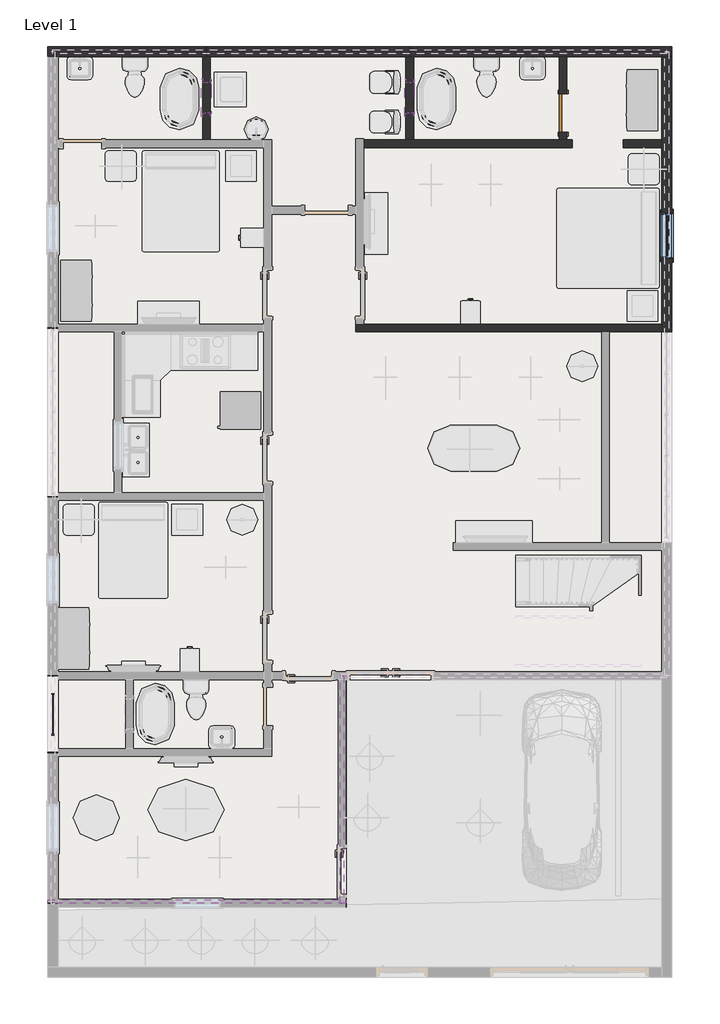
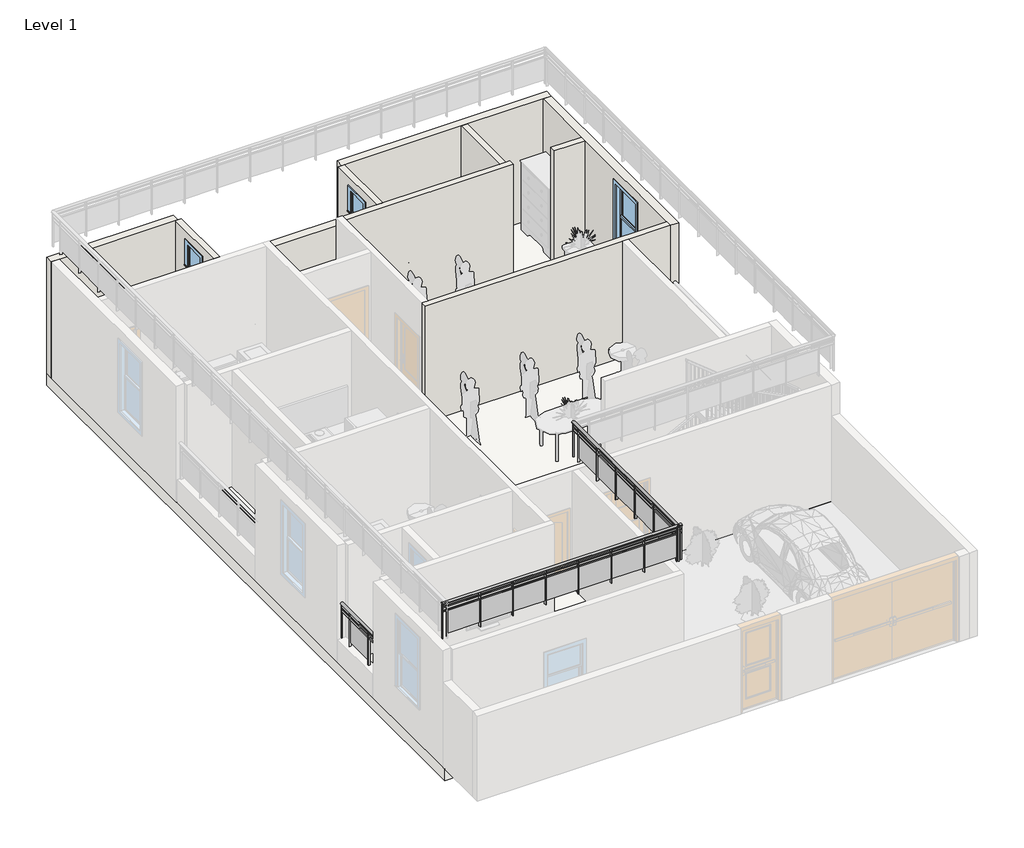
# One storey, part 2 of 6: 10 walls, 3 railings, 3 windows, 1 door, 1 slab.
"""IFC4 building model written with IfcOpenShell, lengths in millimetres."""

from ifc_helpers import new_model, si_unit, point, frame, origin, origin_with_axes, place, context, project, spatial, polyline, ellipse_curve, trimmed, outline, extrude, faceted_brep, transform, mapped, element, save
from ifc_brep_helpers import plane_surface, extruded_surface, advanced_brep
from components import door_255cab33, window_d3583dd1, window_3d781103

model = new_model("IFC4")

# Units and contexts
model_context = context("Model", 3, world=origin())
ifc_project = project(units=[si_unit("LENGTHUNIT", "METRE", prefix="MILLI")], contexts=[model_context])

# Site, building, storey
site = spatial("IfcSite", under=ifc_project)
building = spatial("IfcBuilding", under=site)
storey = spatial("IfcBuildingStorey", under=building, Name="Level 1", Elevation=0.0)

# Door
placement = place(None, origin())
door_shape = door_255cab33(model_context)
element("IfcDoor", 1, ObjectType="Single-Flush : 30\" x 80\"", at=placement, inside=storey, context=model_context, shape_type="MappedRepresentation", body=[
    mapped(door_shape, transform((-4370.9841185, 12532.4271763, 0.0), x_axis=(0.0, -1.0, 0.0), y_axis=(1.0, 0.0, 0.0), z_axis=(0.0, 0.0, 1.0))),
])

# Railings
element("IfcRailing", 2, ObjectType="Glass Panel - Bottom Fill", at=placement, inside=storey, context=model_context, shape_type="SolidModel", body=[
    advanced_brep(
    [(-14467.4841185, 1356.4271763, 1524.0), (-14543.6841185, 1356.4271763, 1524.0), (-14467.4841185, -180.2728237, 1524.0), (-14543.6841185, -180.2728237, 1524.0)],
    [
        (0, 1, ellipse_curve(frame((-14505.5841185, 1356.4271763, 1524.0), z_axis=(0.0, 1.0, 0.0), x_axis=(-1.0, 0.0, 0.0)), 38.1, 28.575)),
        (1, 0, ellipse_curve(frame((-14505.5841185, 1356.4271763, 1524.0), z_axis=(0.0, 1.0, 0.0), x_axis=(-1.0, 0.0, 0.0)), 38.1, 28.575)),
        (2, 3, ellipse_curve(frame((-14505.5841185, -180.2728237, 1524.0), z_axis=(0.0, -1.0, 0.0), x_axis=(-1.0, 0.0, 0.0)), 38.1, 28.575)),
        (3, 2, ellipse_curve(frame((-14505.5841185, -180.2728237, 1524.0), z_axis=(0.0, -1.0, 0.0), x_axis=(-1.0, 0.0, 0.0)), 38.1, 28.575)),
        (0, 2),
        (3, 1),
    ],
    [
        plane_surface(frame((-14505.5841185, 1356.4271763, 1524.0), z_axis=(0.0, 1.0, 0.0), x_axis=(0.0, 0.0, -1.0))),
        plane_surface(frame((-14505.5841185, -180.2728237, 1524.0), z_axis=(0.0, -1.0, 0.0), x_axis=(0.0, 0.0, -1.0))),
        extruded_surface(trimmed(ellipse_curve(frame((-14505.5841185, -180.2728237, 1524.0), z_axis=(0.0, 1.0, 0.0), x_axis=(-1.0, 0.0, 0.0)), 38.1, 28.575), [point((-14467.4841185, -180.2728237, 1524.0))], [point((-14543.6841185, -180.2728237, 1524.0))], True, "CARTESIAN"), (0.0, 1536.6999999999998, 0.0), 1536.6999999999998),
        extruded_surface(trimmed(ellipse_curve(frame((-14505.5841185, -180.2728237, 1524.0), z_axis=(0.0, 1.0, 0.0), x_axis=(-1.0, 0.0, 0.0)), 38.1, 28.575), [point((-14543.6841185, -180.2728237, 1524.0))], [point((-14467.4841185, -180.2728237, 1524.0))], True, "CARTESIAN"), (0.0, 1536.6999999999998, 0.0), 1536.6999999999998),
    ],
    [
        (0, [[1, 2]]),
        (1, [[3, 4]]),
        (2, [[-1, 5, -4, 6]]),
        (3, [[-2, -6, -3, -5]]),
    ],
),
    extrude(outline(polyline([(-14518.2841185, 1356.4271763), (-14492.8841185, 1356.4271763), (-14492.8841185, -180.2728237), (-14518.2841185, -180.2728237), (-14518.2841185, 1356.4271763)])), frame((0.0, 0.0, 1409.7), z_axis=(0.0, 0.0, 1.0), x_axis=(1.0, 0.0, 0.0)), (0.0, 0.0, 1.0), 25.4),
    extrude(outline(polyline([(-14518.2841185, 1356.4271763), (-14492.8841185, 1356.4271763), (-14492.8841185, -180.2728237), (-14518.2841185, -180.2728237), (-14518.2841185, 1356.4271763)])), frame((0.0, 0.0, 1308.1), z_axis=(0.0, 0.0, 1.0), x_axis=(1.0, 0.0, 0.0)), (0.0, 0.0, 1.0), 25.4),
    extrude(outline(polyline([(-14530.9841185, 188.0271763), (-14480.1841185, 188.0271763), (-14480.1841185, 175.3271763), (-14530.9841185, 175.3271763), (-14530.9841185, 188.0271763)])), frame((0.0, 0.0, 609.6), z_axis=(0.0, 0.0, 1.0), x_axis=(1.0, 0.0, 0.0)), (0.0, 0.0, 1.0), 885.6788223),
    extrude(outline(polyline([(-14499.0489615, 994.4771763), (-14499.0489615, 181.6771763), (-14505.3989615, 181.6771763), (-14505.3989615, 994.4771763), (-14499.0489615, 994.4771763)])), frame((0.0, 0.0, 711.2), z_axis=(0.0, 0.0, 1.0), x_axis=(1.0, 0.0, 0.0)), (0.0, 0.0, 1.0), 596.9),
    extrude(outline(polyline([(-14530.9841185, 1000.8271763), (-14480.1841185, 1000.8271763), (-14480.1841185, 988.1271763), (-14530.9841185, 988.1271763), (-14530.9841185, 1000.8271763)])), frame((0.0, 0.0, 609.6), z_axis=(0.0, 0.0, 1.0), x_axis=(1.0, 0.0, 0.0)), (0.0, 0.0, 1.0), 885.6788223),
    extrude(outline(polyline([(-14515.1091185, -167.5728237), (-14496.0591185, -167.5728237), (-14496.0591185, -186.6228237), (-14515.1091185, -186.6228237), (-14515.1091185, -167.5728237)])), frame((0.0, 0.0, 609.6), z_axis=(0.0, 0.0, 1.0), x_axis=(1.0, 0.0, 0.0)), (0.0, 0.0, 1.0), 885.6788223),
    extrude(outline(polyline([(-14515.1091185, 1362.7771763), (-14496.0591185, 1362.7771763), (-14496.0591185, 1343.7271763), (-14515.1091185, 1343.7271763), (-14515.1091185, 1362.7771763)])), frame((0.0, 0.0, 609.6), z_axis=(0.0, 0.0, 1.0), x_axis=(1.0, 0.0, 0.0)), (0.0, 0.0, 1.0), 885.6788223),
])
element("IfcRailing", 3, ObjectType="Glass Panel - Bottom Fill", at=placement, inside=storey, context=model_context, shape_type="SolidModel", body=[
    advanced_brep(
    [(-8727.0841185, 1356.4271763, 4267.2), (-8803.2841185, 1356.4271763, 4267.2), (-8727.0841185, -3164.7728237, 4267.2), (-8803.2841185, -3164.7728237, 4267.2)],
    [
        (0, 1, ellipse_curve(frame((-8765.1841185, 1356.4271763, 4267.2), z_axis=(0.0, 1.0, 0.0), x_axis=(-1.0, 0.0, 0.0)), 38.1, 28.575)),
        (1, 0, ellipse_curve(frame((-8765.1841185, 1356.4271763, 4267.2), z_axis=(0.0, 1.0, 0.0), x_axis=(-1.0, 0.0, 0.0)), 38.1, 28.575)),
        (2, 3, ellipse_curve(frame((-8765.1841185, -3164.7728237, 4267.2), z_axis=(0.0, -1.0, 0.0), x_axis=(-1.0, 0.0, 0.0)), 38.1, 28.575)),
        (3, 2, ellipse_curve(frame((-8765.1841185, -3164.7728237, 4267.2), z_axis=(0.0, -1.0, 0.0), x_axis=(-1.0, 0.0, 0.0)), 38.1, 28.575)),
        (0, 2),
        (3, 1),
    ],
    [
        plane_surface(frame((-8765.1841185, 1356.4271763, 4267.2), z_axis=(0.0, 1.0, 0.0), x_axis=(0.0, 0.0, -1.0))),
        plane_surface(frame((-8765.1841185, -3164.7728237, 4267.2), z_axis=(0.0, -1.0, 0.0), x_axis=(0.0, 0.0, -1.0))),
        extruded_surface(trimmed(ellipse_curve(frame((-8765.1841185, -3164.7728237, 4267.2), z_axis=(0.0, 1.0, 0.0), x_axis=(-1.0, 0.0, 0.0)), 38.1, 28.575), [point((-8727.0841185, -3164.7728237, 4267.2))], [point((-8803.2841185, -3164.7728237, 4267.2))], True, "CARTESIAN"), (0.0, 4521.2, 0.0), 4521.2),
        extruded_surface(trimmed(ellipse_curve(frame((-8765.1841185, -3164.7728237, 4267.2), z_axis=(0.0, 1.0, 0.0), x_axis=(-1.0, 0.0, 0.0)), 38.1, 28.575), [point((-8803.2841185, -3164.7728237, 4267.2))], [point((-8727.0841185, -3164.7728237, 4267.2))], True, "CARTESIAN"), (0.0, 4521.2, 0.0), 4521.2),
    ],
    [
        (0, [[1, 2]]),
        (1, [[3, 4]]),
        (2, [[-1, 5, -4, 6]]),
        (3, [[-2, -6, -3, -5]]),
    ],
),
    extrude(outline(polyline([(-8777.8841185, 1356.4271763), (-8752.4841185, 1356.4271763), (-8752.4841185, -3164.7728237), (-8777.8841185, -3164.7728237), (-8777.8841185, 1356.4271763)])), frame((0.0, 0.0, 4152.9), z_axis=(0.0, 0.0, 1.0), x_axis=(1.0, 0.0, 0.0)), (0.0, 0.0, 1.0), 25.4),
    extrude(outline(polyline([(-8777.8841185, 1356.4271763), (-8752.4841185, 1356.4271763), (-8752.4841185, -3164.7728237), (-8777.8841185, -3164.7728237), (-8777.8841185, 1356.4271763)])), frame((0.0, 0.0, 4051.3), z_axis=(0.0, 0.0, 1.0), x_axis=(1.0, 0.0, 0.0)), (0.0, 0.0, 1.0), 25.4),
    extrude(outline(polyline([(-8790.5841185, -2929.8228237), (-8739.7841185, -2929.8228237), (-8739.7841185, -2942.5228237), (-8790.5841185, -2942.5228237), (-8790.5841185, -2929.8228237)])), frame((0.0, 0.0, 3352.8), z_axis=(0.0, 0.0, 1.0), x_axis=(1.0, 0.0, 0.0)), (0.0, 0.0, 1.0), 885.6788223),
    extrude(outline(polyline([(-8758.6489615, -2123.3728237), (-8758.6489615, -2936.1728237), (-8764.9989615, -2936.1728237), (-8764.9989615, -2123.3728237), (-8758.6489615, -2123.3728237)])), frame((0.0, 0.0, 3454.4), z_axis=(0.0, 0.0, 1.0), x_axis=(1.0, 0.0, 0.0)), (0.0, 0.0, 1.0), 596.9),
    extrude(outline(polyline([(-8790.5841185, -2117.0228237), (-8739.7841185, -2117.0228237), (-8739.7841185, -2129.7228237), (-8790.5841185, -2129.7228237), (-8790.5841185, -2117.0228237)])), frame((0.0, 0.0, 3352.8), z_axis=(0.0, 0.0, 1.0), x_axis=(1.0, 0.0, 0.0)), (0.0, 0.0, 1.0), 885.6788223),
    extrude(outline(polyline([(-8758.6489615, -1310.5728237), (-8758.6489615, -2123.3728237), (-8764.9989615, -2123.3728237), (-8764.9989615, -1310.5728237), (-8758.6489615, -1310.5728237)])), frame((0.0, 0.0, 3454.4), z_axis=(0.0, 0.0, 1.0), x_axis=(1.0, 0.0, 0.0)), (0.0, 0.0, 1.0), 596.9),
    extrude(outline(polyline([(-8790.5841185, -1304.2228237), (-8739.7841185, -1304.2228237), (-8739.7841185, -1316.9228237), (-8790.5841185, -1316.9228237), (-8790.5841185, -1304.2228237)])), frame((0.0, 0.0, 3352.8), z_axis=(0.0, 0.0, 1.0), x_axis=(1.0, 0.0, 0.0)), (0.0, 0.0, 1.0), 885.6788223),
    extrude(outline(polyline([(-8758.6489615, -497.7728237), (-8758.6489615, -1310.5728237), (-8764.9989615, -1310.5728237), (-8764.9989615, -497.7728237), (-8758.6489615, -497.7728237)])), frame((0.0, 0.0, 3454.4), z_axis=(0.0, 0.0, 1.0), x_axis=(1.0, 0.0, 0.0)), (0.0, 0.0, 1.0), 596.9),
    extrude(outline(polyline([(-8790.5841185, -491.4228237), (-8739.7841185, -491.4228237), (-8739.7841185, -504.1228237), (-8790.5841185, -504.1228237), (-8790.5841185, -491.4228237)])), frame((0.0, 0.0, 3352.8), z_axis=(0.0, 0.0, 1.0), x_axis=(1.0, 0.0, 0.0)), (0.0, 0.0, 1.0), 885.6788223),
    extrude(outline(polyline([(-8758.6489615, 315.0271763), (-8758.6489615, -497.7728237), (-8764.9989615, -497.7728237), (-8764.9989615, 315.0271763), (-8758.6489615, 315.0271763)])), frame((0.0, 0.0, 3454.4), z_axis=(0.0, 0.0, 1.0), x_axis=(1.0, 0.0, 0.0)), (0.0, 0.0, 1.0), 596.9),
    extrude(outline(polyline([(-8790.5841185, 321.3771763), (-8739.7841185, 321.3771763), (-8739.7841185, 308.6771763), (-8790.5841185, 308.6771763), (-8790.5841185, 321.3771763)])), frame((0.0, 0.0, 3352.8), z_axis=(0.0, 0.0, 1.0), x_axis=(1.0, 0.0, 0.0)), (0.0, 0.0, 1.0), 885.6788223),
    extrude(outline(polyline([(-8758.6489615, 1127.8271763), (-8758.6489615, 315.0271763), (-8764.9989615, 315.0271763), (-8764.9989615, 1127.8271763), (-8758.6489615, 1127.8271763)])), frame((0.0, 0.0, 3454.4), z_axis=(0.0, 0.0, 1.0), x_axis=(1.0, 0.0, 0.0)), (0.0, 0.0, 1.0), 596.9),
    extrude(outline(polyline([(-8790.5841185, 1134.1771763), (-8739.7841185, 1134.1771763), (-8739.7841185, 1121.4771763), (-8790.5841185, 1121.4771763), (-8790.5841185, 1134.1771763)])), frame((0.0, 0.0, 3352.8), z_axis=(0.0, 0.0, 1.0), x_axis=(1.0, 0.0, 0.0)), (0.0, 0.0, 1.0), 885.6788223),
    extrude(outline(polyline([(-8774.7091185, -3152.0728237), (-8755.6591185, -3152.0728237), (-8755.6591185, -3171.1228237), (-8774.7091185, -3171.1228237), (-8774.7091185, -3152.0728237)])), frame((0.0, 0.0, 3352.8), z_axis=(0.0, 0.0, 1.0), x_axis=(1.0, 0.0, 0.0)), (0.0, 0.0, 1.0), 885.6788223),
    extrude(outline(polyline([(-8774.7091185, 1362.7771763), (-8755.6591185, 1362.7771763), (-8755.6591185, 1343.7271763), (-8774.7091185, 1343.7271763), (-8774.7091185, 1362.7771763)])), frame((0.0, 0.0, 3352.8), z_axis=(0.0, 0.0, 1.0), x_axis=(1.0, 0.0, 0.0)), (0.0, 0.0, 1.0), 885.6788223),
])
element("IfcRailing", 4, ObjectType="Glass Panel - Bottom Fill", at=placement, inside=storey, context=model_context, shape_type="SolidModel", body=[
    advanced_brep(
    [(-8682.6341185, -3167.7131786, 4267.2), (-8682.6341185, -3091.5131786, 4267.2), (-14607.1841185, -3167.7131786, 4267.2), (-14607.1841185, -3091.5131786, 4267.2)],
    [
        (0, 1, ellipse_curve(frame((-8682.6341185, -3129.6131786, 4267.2), z_axis=(1.0, 0.0, 0.0), x_axis=(0.0, 1.0, 0.0)), 38.1, 28.575)),
        (1, 0, ellipse_curve(frame((-8682.6341185, -3129.6131786, 4267.2), z_axis=(1.0, 0.0, 0.0), x_axis=(0.0, 1.0, 0.0)), 38.1, 28.575)),
        (2, 3, ellipse_curve(frame((-14607.1841185, -3129.6131786, 4267.2), z_axis=(-1.0, 0.0, 0.0), x_axis=(0.0, 1.0, 0.0)), 38.1, 28.575)),
        (3, 2, ellipse_curve(frame((-14607.1841185, -3129.6131786, 4267.2), z_axis=(-1.0, 0.0, 0.0), x_axis=(0.0, 1.0, 0.0)), 38.1, 28.575)),
        (0, 2),
        (3, 1),
    ],
    [
        plane_surface(frame((-8682.6341185, -3129.6131786, 4267.2), z_axis=(1.0, 0.0, 0.0), x_axis=(0.0, -1.0, 0.0))),
        plane_surface(frame((-14607.1841185, -3129.6131786, 4267.2), z_axis=(-1.0, 0.0, 0.0), x_axis=(0.0, -1.0, 0.0))),
        extruded_surface(trimmed(ellipse_curve(frame((-14607.1841185, -3129.6131786, 4267.2), z_axis=(1.0, 0.0, 0.0), x_axis=(0.0, 1.0, 0.0)), 38.1, 28.575), [point((-14607.1841185, -3167.7131786, 4267.2))], [point((-14607.1841185, -3091.5131786, 4267.2))], True, "CARTESIAN"), (5924.549999999999, 0.0, 0.0), 5924.549999999999),
        extruded_surface(trimmed(ellipse_curve(frame((-14607.1841185, -3129.6131786, 4267.2), z_axis=(1.0, 0.0, 0.0), x_axis=(0.0, 1.0, 0.0)), 38.1, 28.575), [point((-14607.1841185, -3091.5131786, 4267.2))], [point((-14607.1841185, -3167.7131786, 4267.2))], True, "CARTESIAN"), (5924.549999999999, 0.0, 0.0), 5924.549999999999),
    ],
    [
        (0, [[1, 2]]),
        (1, [[3, 4]]),
        (2, [[-1, 5, -4, 6]]),
        (3, [[-2, -6, -3, -5]]),
    ],
),
    extrude(outline(polyline([(-8682.6341185, -3116.9131786), (-8682.6341185, -3142.3131786), (-14607.1841185, -3142.3131786), (-14607.1841185, -3116.9131786), (-8682.6341185, -3116.9131786)])), frame((0.0, 0.0, 4152.9), z_axis=(0.0, 0.0, 1.0), x_axis=(1.0, 0.0, 0.0)), (0.0, 0.0, 1.0), 25.4),
    extrude(outline(polyline([(-8682.6341185, -3116.9131786), (-8682.6341185, -3142.3131786), (-14607.1841185, -3142.3131786), (-14607.1841185, -3116.9131786), (-8682.6341185, -3116.9131786)])), frame((0.0, 0.0, 4051.3), z_axis=(0.0, 0.0, 1.0), x_axis=(1.0, 0.0, 0.0)), (0.0, 0.0, 1.0), 25.4),
    extrude(outline(polyline([(-14483.3591185, -3104.2131786), (-14483.3591185, -3155.0131786), (-14496.0591185, -3155.0131786), (-14496.0591185, -3104.2131786), (-14483.3591185, -3104.2131786)])), frame((0.0, 0.0, 3352.8), z_axis=(0.0, 0.0, 1.0), x_axis=(1.0, 0.0, 0.0)), (0.0, 0.0, 1.0), 885.6788223),
    extrude(outline(polyline([(-13676.9091185, -3136.1483356), (-14489.7091185, -3136.1483356), (-14489.7091185, -3129.7983356), (-13676.9091185, -3129.7983356), (-13676.9091185, -3136.1483356)])), frame((0.0, 0.0, 3454.4), z_axis=(0.0, 0.0, 1.0), x_axis=(1.0, 0.0, 0.0)), (0.0, 0.0, 1.0), 596.9),
    extrude(outline(polyline([(-13670.5591185, -3104.2131786), (-13670.5591185, -3155.0131786), (-13683.2591185, -3155.0131786), (-13683.2591185, -3104.2131786), (-13670.5591185, -3104.2131786)])), frame((0.0, 0.0, 3352.8), z_axis=(0.0, 0.0, 1.0), x_axis=(1.0, 0.0, 0.0)), (0.0, 0.0, 1.0), 885.6788223),
    extrude(outline(polyline([(-12864.1091185, -3136.1483356), (-13676.9091185, -3136.1483356), (-13676.9091185, -3129.7983356), (-12864.1091185, -3129.7983356), (-12864.1091185, -3136.1483356)])), frame((0.0, 0.0, 3454.4), z_axis=(0.0, 0.0, 1.0), x_axis=(1.0, 0.0, 0.0)), (0.0, 0.0, 1.0), 596.9),
    extrude(outline(polyline([(-12857.7591185, -3104.2131786), (-12857.7591185, -3155.0131786), (-12870.4591185, -3155.0131786), (-12870.4591185, -3104.2131786), (-12857.7591185, -3104.2131786)])), frame((0.0, 0.0, 3352.8), z_axis=(0.0, 0.0, 1.0), x_axis=(1.0, 0.0, 0.0)), (0.0, 0.0, 1.0), 885.6788223),
    extrude(outline(polyline([(-12051.3091185, -3136.1483356), (-12864.1091185, -3136.1483356), (-12864.1091185, -3129.7983356), (-12051.3091185, -3129.7983356), (-12051.3091185, -3136.1483356)])), frame((0.0, 0.0, 3454.4), z_axis=(0.0, 0.0, 1.0), x_axis=(1.0, 0.0, 0.0)), (0.0, 0.0, 1.0), 596.9),
    extrude(outline(polyline([(-12044.9591185, -3104.2131786), (-12044.9591185, -3155.0131786), (-12057.6591185, -3155.0131786), (-12057.6591185, -3104.2131786), (-12044.9591185, -3104.2131786)])), frame((0.0, 0.0, 3352.8), z_axis=(0.0, 0.0, 1.0), x_axis=(1.0, 0.0, 0.0)), (0.0, 0.0, 1.0), 885.6788223),
    extrude(outline(polyline([(-11238.5091185, -3136.1483356), (-12051.3091185, -3136.1483356), (-12051.3091185, -3129.7983356), (-11238.5091185, -3129.7983356), (-11238.5091185, -3136.1483356)])), frame((0.0, 0.0, 3454.4), z_axis=(0.0, 0.0, 1.0), x_axis=(1.0, 0.0, 0.0)), (0.0, 0.0, 1.0), 596.9),
    extrude(outline(polyline([(-11232.1591185, -3104.2131786), (-11232.1591185, -3155.0131786), (-11244.8591185, -3155.0131786), (-11244.8591185, -3104.2131786), (-11232.1591185, -3104.2131786)])), frame((0.0, 0.0, 3352.8), z_axis=(0.0, 0.0, 1.0), x_axis=(1.0, 0.0, 0.0)), (0.0, 0.0, 1.0), 885.6788223),
    extrude(outline(polyline([(-10425.7091185, -3136.1483356), (-11238.5091185, -3136.1483356), (-11238.5091185, -3129.7983356), (-10425.7091185, -3129.7983356), (-10425.7091185, -3136.1483356)])), frame((0.0, 0.0, 3454.4), z_axis=(0.0, 0.0, 1.0), x_axis=(1.0, 0.0, 0.0)), (0.0, 0.0, 1.0), 596.9),
    extrude(outline(polyline([(-10419.3591185, -3104.2131786), (-10419.3591185, -3155.0131786), (-10432.0591185, -3155.0131786), (-10432.0591185, -3104.2131786), (-10419.3591185, -3104.2131786)])), frame((0.0, 0.0, 3352.8), z_axis=(0.0, 0.0, 1.0), x_axis=(1.0, 0.0, 0.0)), (0.0, 0.0, 1.0), 885.6788223),
    extrude(outline(polyline([(-9612.9091185, -3136.1483356), (-10425.7091185, -3136.1483356), (-10425.7091185, -3129.7983356), (-9612.9091185, -3129.7983356), (-9612.9091185, -3136.1483356)])), frame((0.0, 0.0, 3454.4), z_axis=(0.0, 0.0, 1.0), x_axis=(1.0, 0.0, 0.0)), (0.0, 0.0, 1.0), 596.9),
    extrude(outline(polyline([(-9606.5591185, -3104.2131786), (-9606.5591185, -3155.0131786), (-9619.2591185, -3155.0131786), (-9619.2591185, -3104.2131786), (-9606.5591185, -3104.2131786)])), frame((0.0, 0.0, 3352.8), z_axis=(0.0, 0.0, 1.0), x_axis=(1.0, 0.0, 0.0)), (0.0, 0.0, 1.0), 885.6788223),
    extrude(outline(polyline([(-8800.1091185, -3136.1483356), (-9612.9091185, -3136.1483356), (-9612.9091185, -3129.7983356), (-8800.1091185, -3129.7983356), (-8800.1091185, -3136.1483356)])), frame((0.0, 0.0, 3454.4), z_axis=(0.0, 0.0, 1.0), x_axis=(1.0, 0.0, 0.0)), (0.0, 0.0, 1.0), 596.9),
    extrude(outline(polyline([(-8793.7591185, -3104.2131786), (-8793.7591185, -3155.0131786), (-8806.4591185, -3155.0131786), (-8806.4591185, -3104.2131786), (-8793.7591185, -3104.2131786)])), frame((0.0, 0.0, 3352.8), z_axis=(0.0, 0.0, 1.0), x_axis=(1.0, 0.0, 0.0)), (0.0, 0.0, 1.0), 885.6788223),
    extrude(outline(polyline([(-14594.4841185, -3120.0881786), (-14594.4841185, -3139.1381786), (-14613.5341185, -3139.1381786), (-14613.5341185, -3120.0881786), (-14594.4841185, -3120.0881786)])), frame((0.0, 0.0, 3352.8), z_axis=(0.0, 0.0, 1.0), x_axis=(1.0, 0.0, 0.0)), (0.0, 0.0, 1.0), 885.6788223),
    extrude(outline(polyline([(-8676.2841185, -3120.0881786), (-8676.2841185, -3139.1381786), (-8695.3341185, -3139.1381786), (-8695.3341185, -3120.0881786), (-8676.2841185, -3120.0881786)])), frame((0.0, 0.0, 3352.8), z_axis=(0.0, 0.0, 1.0), x_axis=(1.0, 0.0, 0.0)), (0.0, 0.0, 1.0), 885.6788223),
])

# Slab
element("IfcSlab", 5, ObjectType="Generic - 12\"", at=placement, inside=storey, context=model_context, shape_type="SweptSolid", body=[
    extrude(outline(polyline([(-2211.9841185, 13853.2271763), (-2211.9841185, 1280.2271763), (-8682.6341185, 1280.2271763), (-8682.6341185, -3240.9728237), (-14607.1841185, -3240.9728237), (-14607.1841185, 13853.2271763), (-2211.9841185, 13853.2271763)])), frame((0.0, 0.0, -304.8), z_axis=(0.0, 0.0, 1.0), x_axis=(1.0, 0.0, 0.0)), (0.0, 0.0, 1.0), 304.8),
])

# Walls
element("IfcWall", 6, ObjectType="Generic - 8\"", at=placement, inside=storey, context=model_context, shape_type="Brep", body=[
    faceted_brep([(-14607.1841185, 13650.0271763, 0.0), (-14403.9841185, 13650.0271763, 0.0), (-11470.2841185, 13650.0271763, 0.0), (-11470.2841185, 13650.0271763, 3048.0), (-14403.9841185, 13650.0271763, 3048.0), (-14607.1841185, 13650.0271763, 3048.0), (-14607.1841185, 13853.2271763, 0.0), (-14607.1841185, 13853.2271763, 3048.0), (-11470.2841185, 13853.2271763, 3048.0), (-11470.2841185, 13853.2271763, 0.0)], [[[0, 1, 2, 3, 4, 5]], [[6, 7, 8, 9]], [[2, 1, 0, 6, 9]], [[3, 2, 9, 8]], [[0, 5, 7, 6]], [[5, 4, 3, 8, 7]]]),
])
element("IfcWall", 7, ObjectType="Generic - 8\"", at=placement, inside=storey, context=model_context, shape_type="Brep", body=[
    faceted_brep([(-2415.1841185, 13650.0271763, 0.0), (-2415.1841185, 11999.0271763, 0.0), (-2415.1841185, 11846.6271763, 0.0), (-2415.1841185, 8341.4271763, 0.0), (-2415.1841185, 8265.2271763, 0.0), (-2415.1841185, 8265.2271763, 609.6), (-2415.1841185, 8189.0271763, 609.6), (-2415.1841185, 8189.0271763, 3048.0), (-2415.1841185, 8341.4271763, 3048.0), (-2415.1841185, 11846.6271763, 3048.0), (-2415.1841185, 11999.0271763, 3048.0), (-2415.1841185, 13650.0271763, 3048.0), (-2415.1841185, 9636.8271763, 2743.2), (-2415.1841185, 9636.8271763, 914.4), (-2415.1841185, 10551.2271763, 914.4), (-2415.1841185, 10551.2271763, 2743.2), (-2211.9841185, 13650.0271763, 0.0), (-2211.9841185, 13650.0271763, 3048.0), (-2211.9841185, 8189.0271763, 3048.0), (-2211.9841185, 8189.0271763, 609.6), (-2211.9841185, 8265.2271763, 609.6), (-2211.9841185, 8265.2271763, 0.0), (-2211.9841185, 9636.8271763, 2743.2), (-2211.9841185, 10551.2271763, 2743.2), (-2211.9841185, 10551.2271763, 914.4), (-2211.9841185, 9636.8271763, 914.4)], [[[0, 1, 2, 3, 4, 5, 6, 7, 8, 9, 10, 11], [12, 13, 14, 15]], [[16, 17, 18, 19, 20, 21], [22, 23, 24, 25]], [[4, 3, 2, 1, 0, 16, 21]], [[0, 11, 17, 16]], [[13, 12, 22, 25]], [[14, 13, 25, 24]], [[15, 14, 24, 23]], [[12, 15, 23, 22]], [[5, 4, 21, 20]], [[19, 6, 5, 20]], [[7, 6, 19, 18]], [[11, 10, 9, 8, 7, 18, 17]]]),
])
element("IfcWall", 8, ObjectType="Generic - 8\"", at=placement, inside=storey, context=model_context, shape_type="Brep", body=[
    faceted_brep([(-7406.2841185, 13650.0271763, 0.0), (-7342.7841185, 13650.0271763, 0.0), (-4447.1841185, 13650.0271763, 0.0), (-4294.7841185, 13650.0271763, 0.0), (-2415.1841185, 13650.0271763, 0.0), (-2211.9841185, 13650.0271763, 0.0), (-2211.9841185, 13650.0271763, 3048.0), (-2415.1841185, 13650.0271763, 3048.0), (-4294.7841185, 13650.0271763, 3048.0), (-4447.1841185, 13650.0271763, 3048.0), (-7342.7841185, 13650.0271763, 3048.0), (-7406.2841185, 13650.0271763, 3048.0), (-7406.2841185, 13853.2271763, 0.0), (-7406.2841185, 13853.2271763, 3048.0), (-2211.9841185, 13853.2271763, 3048.0), (-2211.9841185, 13853.2271763, 0.0)], [[[0, 1, 2, 3, 4, 5, 6, 7, 8, 9, 10, 11]], [[12, 13, 14, 15]], [[5, 4, 3, 2, 1, 0, 12, 15]], [[0, 11, 13, 12]], [[6, 5, 15, 14]], [[11, 10, 9, 8, 7, 6, 14, 13]]]),
])
element("IfcWall", 9, ObjectType="Generic - 8\"", at=placement, inside=storey, context=model_context, shape_type="Brep", body=[
    faceted_brep([(-11444.8841185, 13650.0271763, 0.0), (-11381.3841185, 13650.0271763, 0.0), (-7431.6841185, 13650.0271763, 0.0), (-7431.6841185, 13650.0271763, 1524.0), (-11444.8841185, 13650.0271763, 1524.0), (-11444.8841185, 13853.2271763, 0.0), (-11444.8841185, 13853.2271763, 1524.0), (-7431.6841185, 13853.2271763, 1524.0), (-7431.6841185, 13853.2271763, 0.0)], [[[0, 1, 2, 3, 4]], [[5, 6, 7, 8]], [[2, 1, 0, 5, 8]], [[3, 2, 8, 7]], [[4, 3, 7, 6]], [[0, 4, 6, 5]]]),
])
element("IfcWall", 10, ObjectType="INNER -6\"", at=placement, inside=storey, context=model_context, shape_type="Brep", body=[
    faceted_brep([(-11381.3841185, 11999.0271763, 0.0), (-11381.3841185, 13650.0271763, 0.0), (-11381.3841185, 13650.0271763, 3048.0), (-11381.3841185, 11999.0271763, 3048.0), (-11381.3841185, 13142.0271763, 2768.6), (-11381.3841185, 13142.0271763, 2159.0), (-11381.3841185, 12532.4271763, 2159.0), (-11381.3841185, 12532.4271763, 2768.6), (-11533.7841185, 11999.0271763, 0.0), (-11533.7841185, 11999.0271763, 3048.0), (-11533.7841185, 13650.0271763, 3048.0), (-11533.7841185, 13650.0271763, 0.0), (-11533.7841185, 13142.0271763, 2768.6), (-11533.7841185, 12532.4271763, 2768.6), (-11533.7841185, 12532.4271763, 2159.0), (-11533.7841185, 13142.0271763, 2159.0), (-11444.8841185, 13650.0271763, 0.0)], [[[0, 1, 2, 3], [4, 5, 6, 7]], [[8, 9, 10, 11], [12, 13, 14, 15]], [[1, 0, 8, 11, 16]], [[0, 3, 9, 8]], [[2, 1, 16, 11, 10]], [[5, 4, 12, 15]], [[6, 5, 15, 14]], [[7, 6, 14, 13]], [[4, 7, 13, 12]], [[3, 2, 10, 9]]]),
])
element("IfcWall", 11, ObjectType="INNER -6\"", at=placement, inside=storey, context=model_context, shape_type="Brep", body=[
    faceted_brep([(-8333.3841185, 11846.6271763, 0.0), (-4193.1841185, 11846.6271763, 0.0), (-4193.1841185, 11846.6271763, 3048.0), (-8333.3841185, 11846.6271763, 3048.0), (-8333.3841185, 11999.0271763, 0.0), (-8333.3841185, 11999.0271763, 3048.0), (-7495.1841185, 11999.0271763, 3048.0), (-7342.7841185, 11999.0271763, 3048.0), (-4447.1841185, 11999.0271763, 3048.0), (-4294.7841185, 11999.0271763, 3048.0), (-4193.1841185, 11999.0271763, 3048.0), (-4193.1841185, 11999.0271763, 0.0), (-4294.7841185, 11999.0271763, 0.0), (-4447.1841185, 11999.0271763, 0.0), (-7342.7841185, 11999.0271763, 0.0), (-7495.1841185, 11999.0271763, 0.0)], [[[0, 1, 2, 3]], [[4, 5, 6, 7, 8, 9, 10, 11, 12, 13, 14, 15]], [[1, 0, 4, 15, 14, 13, 12, 11]], [[2, 1, 11, 10]], [[0, 3, 5, 4]], [[3, 2, 10, 9, 8, 7, 6, 5]]]),
])
element("IfcWall", 12, ObjectType="INNER -6\"", at=placement, inside=storey, context=model_context, shape_type="Brep", body=[
    faceted_brep([(-2415.1841185, 8341.4271763, 3048.0), (-2415.1841185, 8341.4271763, 0.0), (-8333.3841185, 8341.4271763, 0.0), (-8485.7841185, 8341.4271763, 0.0), (-8485.7841185, 8341.4271763, 3048.0), (-8333.3841185, 8341.4271763, 3048.0), (-2415.1841185, 8189.0271763, 0.0), (-2415.1841185, 8189.0271763, 609.6), (-2415.1841185, 8189.0271763, 3048.0), (-3456.5841185, 8189.0271763, 3048.0), (-3608.9841185, 8189.0271763, 3048.0), (-8485.7841185, 8189.0271763, 3048.0), (-8485.7841185, 8189.0271763, 0.0), (-3608.9841185, 8189.0271763, 0.0), (-3456.5841185, 8189.0271763, 0.0), (-2415.1841185, 8265.2271763, 0.0)], [[[0, 1, 2, 3, 4, 5]], [[6, 7, 8, 9, 10, 11, 12, 13, 14]], [[3, 2, 1, 15, 6, 14, 13, 12]], [[4, 3, 12, 11]], [[0, 8, 7, 6, 15, 1]], [[0, 5, 4, 11, 10, 9, 8]]]),
])
element("IfcWall", 13, ObjectType="INNER -6\"", at=placement, inside=storey, context=model_context, shape_type="Brep", body=[
    faceted_brep([(-7495.1841185, 13650.0271763, 0.0), (-7495.1841185, 11999.0271763, 0.0), (-7495.1841185, 11999.0271763, 3048.0), (-7495.1841185, 13650.0271763, 3048.0), (-7495.1841185, 13142.0271763, 2768.6), (-7495.1841185, 12532.4271763, 2768.6), (-7495.1841185, 12532.4271763, 2159.0), (-7495.1841185, 13142.0271763, 2159.0), (-7342.7841185, 13650.0271763, 0.0), (-7342.7841185, 13650.0271763, 3048.0), (-7342.7841185, 11999.0271763, 3048.0), (-7342.7841185, 11999.0271763, 0.0), (-7342.7841185, 13142.0271763, 2768.6), (-7342.7841185, 13142.0271763, 2159.0), (-7342.7841185, 12532.4271763, 2159.0), (-7342.7841185, 12532.4271763, 2768.6), (-7406.2841185, 13650.0271763, 0.0), (-7406.2841185, 13650.0271763, 3048.0)], [[[0, 1, 2, 3], [4, 5, 6, 7]], [[8, 9, 10, 11], [12, 13, 14, 15]], [[1, 0, 16, 8, 11]], [[0, 3, 17, 9, 8, 16]], [[2, 1, 11, 10]], [[13, 12, 4, 7]], [[14, 13, 7, 6]], [[15, 14, 6, 5]], [[12, 15, 5, 4]], [[3, 2, 10, 9, 17]]]),
])
element("IfcWall", 14, ObjectType="INNER -6\"", at=placement, inside=storey, context=model_context, shape_type="SweptSolid", body=[
    extrude(outline(polyline([(12151.4271763, 2032.0), (12151.4271763, 0.0), (11999.0271763, 0.0), (11999.0271763, 3048.0), (13650.0271763, 3048.0), (13650.0271763, 0.0), (12913.4271763, 0.0), (12913.4271763, 2032.0), (12151.4271763, 2032.0)])), frame((-4447.1841185, 0.0, 0.0), z_axis=(1.0, 0.0, 0.0), x_axis=(0.0, 1.0, 0.0)), (0.0, 0.0, 1.0), 152.4),
])
element("IfcWall", 15, ObjectType="INNER -6\"", at=placement, inside=storey, context=model_context, shape_type="SweptSolid", body=[
    extrude(outline(polyline([(-2415.1841185, 11846.6271763), (-3177.1841185, 11846.6271763), (-3177.1841185, 11999.0271763), (-2415.1841185, 11999.0271763), (-2415.1841185, 11846.6271763)])), origin_with_axes(), (0.0, 0.0, 1.0), 3048.0),
])

# Windows
window_shape = window_d3583dd1(model_context)
element("IfcWindow", 16, ObjectType="Double Hung with Trim : 36\" x 72\"", at=placement, inside=storey, context=model_context, shape_type="MappedRepresentation", body=[
    mapped(window_shape, transform((-2313.5841185, 10094.0271763, 609.6), x_axis=(0.0, -1.0, 0.0), y_axis=(1.0, 0.0, 0.0), z_axis=(0.0, 0.0, 1.0))),
])
window_2_shape = window_3d781103(model_context)
element("IfcWindow", 17, ObjectType="Transom with Trim : 24\" x 24\"", at=placement, inside=storey, context=model_context, shape_type="MappedRepresentation", body=[
    mapped(window_2_shape, transform((-11457.5841185, 12875.3271763, 0.0), x_axis=(0.0, 1.0, 0.0), y_axis=(-1.0, 0.0, 0.0), z_axis=(0.0, 0.0, 1.0))),
])
element("IfcWindow", 18, ObjectType="Transom with Trim : 24\" x 24\"", at=placement, inside=storey, context=model_context, shape_type="MappedRepresentation", body=[
    mapped(window_2_shape, transform((-7418.9841185, 12875.3271763, 0.0), x_axis=(0.0, 1.0, 0.0), y_axis=(-1.0, 0.0, 0.0), z_axis=(0.0, 0.0, 1.0))),
])

save(model, "model.ifc")

# Revit data of these elements
# Type "Single-Flush : 30\" x 80\""
#   Type Mark = "5"
#   Construction Type Id = "MDOOR"
#   Assembly Code = "C1020"
#   Analytic Construction = "Metal"
#   Thickness = 0' - 2"
#   Heat Transfer Coefficient (U) = 0.651978 BTU/(h·ft²·°F)
#   Height = 6' - 8"
#   Trim Projection Ext = 0' - 1"
#   Trim Projection Int = 0' - 1"
#   Trim Width = 0' - 3"
#   Width = 2' - 6"
#   Define Thermal Properties by = 1
#   Door Material = Door - Panel
#   Frame Material = Door - Frame
#   Visual Light Transmittance = 0
#   Solar Heat Gain Coefficient = 0
#   Function = (empty or 0)
#   Wall Closure = (empty or 0)
# Type "Glass Panel - Bottom Fill"
#   Assembly Code = "C2010400"
#   built-in parameter 1008612 = 0.0416667 (stored number, unit not read)
#   built-in parameter 1008611 = 0.0416667 (stored number, unit not read)
#   built-in parameter 1008609 = 0.333333 (stored number, unit not read)
#   built-in parameter 1008604 = 0.166667 (stored number, unit not read)
#   built-in parameter 1008603 = 0.166667 (stored number, unit not read)
#   Railing Height = 3' - 0"
#   built-in parameter 1008630 = 2
#   built-in parameter 1008610 = 2
#   built-in parameter 1008618 = Baluster - Square : 3/4"
# Type "Generic - 12\""
#   Assembly Code = "B1010"
#   Function = 0
#   Layers, outside or top first: 1' - 0" no material (function 1)
# Type "Generic - 8\""
#   Assembly Code = "B2010"
#   Layers, outside or top first: 0' - 8" "Brick, Common" (function 1)
# Type "INNER -6\""
#   Assembly Code = "B2010"
#   Layers, outside or top first: 0' - 6" "Brick, Common" (function 1)
# Type "Double Hung with Trim : 36\" x 72\""
#   Type Mark = "18"
#   Construction Type Id = "GSP4R"
#   Assembly Code = "B2020100"
#   Analytic Construction = "1/8 in Pilkington single glazing"
#   Visual Light Transmittance = 0.9
#   Solar Heat Gain Coefficient = 0.78
#   Heat Transfer Coefficient (U) = 0.6496 BTU/(h·ft²·°F)
#   Height = 6' - 0"
#   Default Sill Height = 1' - 0"
#   Trim Projection - Ext. = 0' - 0 1/2"
#   Trim Projection - Int. = 0' - 0 3/4"
#   Trim Width - Exterior = 0' - 3 1/2"
#   Trim Width - Interior = 0' - 3 1/2"
#   Width = 3' - 0"
#   Window Inset = 0' - 0 3/4"
#   Define Thermal Properties by = 1
#   Glass Pane Material = Glass
#   Sash Material = Sash
#   Trim Exterior Material = Trim
#   Trim Interior Material = Trim
#   Wall Closure = (empty or 0)
# Type "Transom with Trim : 24\" x 24\""
#   Type Mark = "19"
#   Construction Type Id = "GSP4R"
#   Assembly Code = "B2020100"
#   Analytic Construction = "1/8 in Pilkington single glazing"
#   Visual Light Transmittance = 0.9
#   Solar Heat Gain Coefficient = 0.78
#   Heat Transfer Coefficient (U) = 0.6496 BTU/(h·ft²·°F)
#   Height = 2' - 0"
#   Default Sill Height = 7' - 1"
#   Trim Projection - Ext. = 0' - 0 1/2"
#   Trim Projection - Int. = 0' - 0 3/4"
#   Trim Width - Exterior = 0' - 3 1/2"
#   Trim Width - Interior = 0' - 3 1/2"
#   Width = 2' - 0"
#   Window Inset = 0' - 0 3/4"
#   Define Thermal Properties by = 1
#   Glass Pane Material = Glass
#   Sash Material = Sash
#   Trim Exterior Material = Trim
#   Trim Interior Material = Trim
#   Wall Closure = (empty or 0)
# Element 1 (IfcDoor, "Single-Flush : 30\" x 80\"")
#   Phase Created = New Construction
#   Materials on its faces: "Door - Frame", "Door - Panel"
# Element 2 (IfcRailing, "Glass Panel - Bottom Fill")
#   built-in parameter 1008621 = 2 (stored number, unit not read)
#   Phase Created = New Construction
#   Materials on its faces: "Glass"
# Elements 3, 4 (IfcRailing, "Glass Panel - Bottom Fill")
#   built-in parameter 1008621 = 11 (stored number, unit not read)
#   Phase Created = New Construction
#   Materials on its faces: "Glass"
# Element 5 (IfcSlab, "Generic - 12\"")
#   Height Offset From Level = 0' - 0"
#   Phase Created = New Construction
#   Materials on its faces: "Default Floor"
# Elements 6, 7, 8 (IfcWall, "Generic - 8\"")
#   Top Offset = 0' - 0"
#   Base Offset = 0' - 0"
#   Unconnected Height = 10' - 0"
#   wall height = 10' - 0"
#   Phase Created = New Construction
#   Base Constraint = Level 1
#   Materials on its faces: "Brick, Common"
# Element 9 (IfcWall, "Generic - 8\"")
#   Top Offset = 0' - 0"
#   Base Offset = 0' - 0"
#   Unconnected Height = 5' - 0"
#   wall height = 5' - 0"
#   Phase Created = New Construction
#   Base Constraint = Level 1
#   Materials on its faces: "Brick, Common"
# Elements 10, 11, 12, 13, 14, 15 (IfcWall, "INNER -6\"")
#   Top Offset = 0' - 0"
#   Base Offset = 0' - 0"
#   Unconnected Height = 10' - 0"
#   wall height = 10' - 0"
#   Phase Created = New Construction
#   Base Constraint = Level 1
#   Materials on its faces: "Brick, Common"
# Element 16 (IfcWindow, "Double Hung with Trim : 36\" x 72\"")
#   Mark = "2"
#   Phase Created = New Construction
#   Materials on its faces: "Sash", "Trim", "Glass"
# Element 17 (IfcWindow, "Transom with Trim : 24\" x 24\"")
#   Mark = "7"
#   Phase Created = New Construction
#   Materials on its faces: "Sash", "Trim", "Glass"
# Element 18 (IfcWindow, "Transom with Trim : 24\" x 24\"")
#   Mark = "8"
#   Phase Created = New Construction
#   Materials on its faces: "Sash", "Trim", "Glass"
# Materials
#   "Door - Panel": class "Wood", colour RGB 210 159 95, transparency 0
#   "Door - Frame": colour RGB 118 70 51, transparency 0
#   "Brick, Common": class "Masonry", colour RGB 170 98 104, transparency 0, Description = "Common brick", Cost = 0
#   "Glass": class "Glass", colour RGB 0 128 192, transparency 0.75, Description = "Soda Lime Glass", Cost = 0
#   "Sash": class "Wood", colour RGB 224 178 126, transparency 0
#   "Trim": class "Wood", colour RGB 224 178 126, transparency 0
#   "Default Floor": colour RGB 128 128 128, transparency 0
